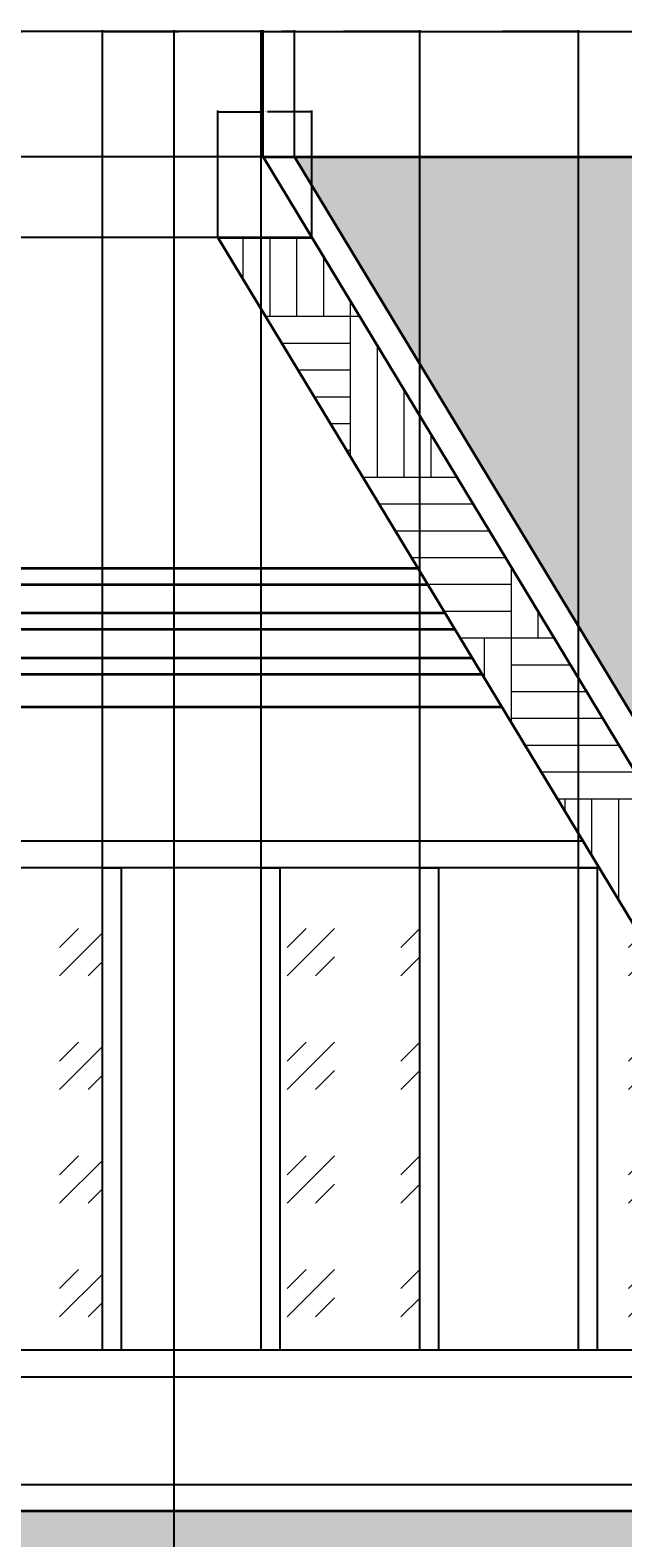
# Model space of a CAD drawing. Units: inches. Extents: x -9 to 389, y -55 to 344.
# Tile 4 of 5: x 133 to 221, y 119 to 344. Entities that reach past the tile are written whole.
import ezdxf

# ---------------------------------------------------------------- set-up
doc = ezdxf.new("R2010")
doc.units = ezdxf.units.IN
doc.header["$MEASUREMENT"] = 0
for name, color, linetype, lineweight in [('A-ANNO-DIMS', 2, 'Continuous', 18), ('A-ELEV', 7, 'Continuous', 35), ('A-ELEV-PATT', 8, 'Continuous', 13), ('A-GLAZ', 4, 'Continuous', 25), ('A-GLAZ-PATT', 252, 'Continuous', 13), ('A-ROOF', 1, 'Continuous', 35), ('A-ROOF-PATT', 8, 'Continuous', 13)]:
    doc.layers.add(name, color=color, linetype=linetype, lineweight=lineweight)
doc.styles.get("Standard").update_dxf_attribs({"font": 'arial.ttf'})
doc.dimstyles.get("Standard").update_dxf_attribs({"dimtxt": 0.18, "dimasz": 0.18, "dimexe": 0.18, "dimexo": 0.0625, "dimgap": 0.09, "dimtad": 0, "dimtih": 1, "dimtoh": 1, "dimdec": 4, "dimzin": 0, "dimdsep": 46, "dimtxsty": 'Standard', "dimcen": 0.09, "dimadec": 0, "dimazin": 0, "dimtfac": 1, "dimtdec": 4, "dimtofl": 0, "dimtmove": 0, "dimatfit": 3, "dimfxl": 1, "dimtolj": 1, "dimtzin": 0, "dimarcsym": 0})

# ---------------------------------------------------------------- blocks, each defined once
blk = doc.blocks.new('*D4')
at = {"layer": 'A-ANNO-DIMS', "color": 0, "lineweight": -2, "transparency": 16777216}
for p, q in [((71.45, 157.47), (71.45, 343.8)), ((71.63, 343.62), (119.03, 343.62)), ((167.08, 343.62), (119.68, 343.62)), ((167.26, 324.93), (167.26, 343.8))]:
    blk.add_line(p, q, dxfattribs=at)
at = {"layer": 'A-ANNO-DIMS', "color": 0, "transparency": 16777216}
for points in [[(71.63, 343.65), (71.63, 343.59), (71.45, 343.62)], [(167.08, 343.65), (167.08, 343.59), (167.26, 343.62)]]:
    blk.add_solid(points, dxfattribs=at)
at = {"layer": 'Defpoints', "color": 0, "transparency": 16777216}
for p in [(167.26, 343.62), (167.26, 324.87), (71.45, 157.4)]:
    blk.add_point(p, dxfattribs=at)
at = {"layer": 'A-ANNO-DIMS', "color": 0, "transparency": 16777216, "insert": (119.35, 343.62), "char_height": 0.18, "attachment_point": 5}
blk.add_mtext('\\A1;95.8', dxfattribs=at)
blk = doc.blocks.new('*D5')
at = {"layer": 'A-ANNO-DIMS', "color": 0, "lineweight": -2, "transparency": 16777216}
for p, q in [((167.26, 324.93), (167.26, 343.8)), ((167.44, 343.62), (169.2, 343.62)), ((171.75, 343.62), (169.99, 343.62)), ((171.93, 324.93), (171.93, 343.8))]:
    blk.add_line(p, q, dxfattribs=at)
at = {"layer": 'A-ANNO-DIMS', "color": 0, "transparency": 16777216}
for points in [[(167.44, 343.65), (167.44, 343.59), (167.26, 343.62)], [(171.75, 343.65), (171.75, 343.59), (171.93, 343.62)]]:
    blk.add_solid(points, dxfattribs=at)
at = {"layer": 'Defpoints', "color": 0, "transparency": 16777216}
for p in [(171.93, 343.62), (167.26, 324.87), (171.93, 324.87)]:
    blk.add_point(p, dxfattribs=at)
at = {"layer": 'A-ANNO-DIMS', "color": 0, "transparency": 16777216, "insert": (169.59, 343.62), "char_height": 0.18, "attachment_point": 5}
blk.add_mtext('\\A1;4.674', dxfattribs=at)
blk = doc.blocks.new('*D6')
at = {"layer": 'A-ANNO-DIMS', "color": 0, "lineweight": -2, "transparency": 16777216}
for p, q in [((171.93, 324.93), (171.93, 343.8)), ((172.11, 343.62), (270.34, 343.62)), ((369.47, 343.62), (271.25, 343.62)), ((369.65, 324.93), (369.65, 343.8))]:
    blk.add_line(p, q, dxfattribs=at)
at = {"layer": 'A-ANNO-DIMS', "color": 0, "transparency": 16777216}
for points in [[(172.11, 343.65), (172.11, 343.59), (171.93, 343.62)], [(369.47, 343.65), (369.47, 343.59), (369.65, 343.62)]]:
    blk.add_solid(points, dxfattribs=at)
at = {"layer": 'Defpoints', "color": 0, "transparency": 16777216}
for p in [(369.65, 343.62), (171.93, 324.87), (369.65, 324.87)]:
    blk.add_point(p, dxfattribs=at)
at = {"layer": 'A-ANNO-DIMS', "color": 0, "transparency": 16777216, "insert": (270.79, 343.62), "char_height": 0.18, "attachment_point": 5}
blk.add_mtext('\\A1;197.72', dxfattribs=at)
blk = doc.blocks.new('*D19')
at = {"layer": 'A-ANNO-DIMS', "color": 0, "lineweight": -2, "transparency": 16777216}
for p, q in [((66.21, 14.83), (66.21, 343.8)), ((66.39, 343.62), (109.71, 343.62)), ((153.81, 343.62), (110.5, 343.62)), ((153.99, 14.83), (153.99, 343.8))]:
    blk.add_line(p, q, dxfattribs=at)
at = {"layer": 'A-ANNO-DIMS', "color": 0, "transparency": 16777216}
for points in [[(66.39, 343.65), (66.39, 343.59), (66.21, 343.62)], [(153.81, 343.65), (153.81, 343.59), (153.99, 343.62)]]:
    blk.add_solid(points, dxfattribs=at)
at = {"layer": 'Defpoints', "color": 0, "transparency": 16777216}
for p in [(153.99, 343.62), (66.21, 14.77), (153.99, 14.77)]:
    blk.add_point(p, dxfattribs=at)
at = {"layer": 'A-ANNO-DIMS', "color": 0, "transparency": 16777216, "insert": (110.1, 343.62), "char_height": 0.18, "attachment_point": 5}
blk.add_mtext('\\A1;87.77', dxfattribs=at)
blk = doc.blocks.new('*D20')
at = {"layer": 'A-ANNO-DIMS', "color": 0, "lineweight": -2, "transparency": 16777216}
for p, q in [((369.72, 324.87), (388.58, 324.87)), ((388.4, 324.69), (388.4, 144.62)), ((388.4, -35.81), (388.4, 144.26)), ((146.92, -35.99), (388.58, -35.99))]:
    blk.add_line(p, q, dxfattribs=at)
at = {"layer": 'A-ANNO-DIMS', "color": 0, "transparency": 16777216}
for points in [[(388.37, 324.69), (388.43, 324.69), (388.4, 324.87)], [(388.37, -35.81), (388.43, -35.81), (388.4, -35.99)]]:
    blk.add_solid(points, dxfattribs=at)
at = {"layer": 'Defpoints', "color": 0, "transparency": 16777216}
for p in [(369.65, 324.87), (388.4, 324.87), (146.86, -35.99)]:
    blk.add_point(p, dxfattribs=at)
at = {"layer": 'A-ANNO-DIMS', "color": 0, "transparency": 16777216, "insert": (388.4, 144.44), "char_height": 0.18, "attachment_point": 5}
blk.add_mtext('\\A1;360.86', dxfattribs=at)
blk = doc.blocks.new('*D28')
at = {"layer": 'A-ANNO-DIMS', "color": 0, "lineweight": -2, "transparency": 16777216}
for p, q in [((160.42, 312.87), (-9.28, 312.87)), ((-9.1, 312.69), (-9.1, 297.72)), ((-9.1, 282.38), (-9.1, 297.35)), ((9.59, 282.2), (-9.28, 282.2))]:
    blk.add_line(p, q, dxfattribs=at)
at = {"layer": 'A-ANNO-DIMS', "color": 0, "transparency": 16777216}
for points in [[(-9.13, 312.69), (-9.07, 312.69), (-9.1, 312.87)], [(-9.13, 282.38), (-9.07, 282.38), (-9.1, 282.2)]]:
    blk.add_solid(points, dxfattribs=at)
at = {"layer": 'Defpoints', "color": 0, "transparency": 16777216}
for p in [(-9.1, 312.87), (160.49, 312.87), (9.65, 282.2)]:
    blk.add_point(p, dxfattribs=at)
at = {"layer": 'A-ANNO-DIMS', "color": 0, "transparency": 16777216, "insert": (-9.1, 297.54), "char_height": 0.18, "attachment_point": 5}
blk.add_mtext('\\A1;30.67', dxfattribs=at)
blk = doc.blocks.new('*D29')
at = {"layer": 'A-ANNO-DIMS', "color": 0, "lineweight": -2, "transparency": 16777216}
for p, q in [((369.59, 324.87), (-9.28, 324.87)), ((-9.1, 324.69), (-9.1, 319.05)), ((-9.1, 313.05), (-9.1, 318.69)), ((160.42, 312.87), (-9.28, 312.87))]:
    blk.add_line(p, q, dxfattribs=at)
at = {"layer": 'A-ANNO-DIMS', "color": 0, "transparency": 16777216}
for points in [[(-9.13, 324.69), (-9.07, 324.69), (-9.1, 324.87)], [(-9.13, 313.05), (-9.07, 313.05), (-9.1, 312.87)]]:
    blk.add_solid(points, dxfattribs=at)
at = {"layer": 'Defpoints', "color": 0, "transparency": 16777216}
for p in [(-9.1, 324.87), (369.65, 324.87), (160.49, 312.87)]:
    blk.add_point(p, dxfattribs=at)
at = {"layer": 'A-ANNO-DIMS', "color": 0, "transparency": 16777216, "insert": (-9.1, 318.87), "char_height": 0.18, "attachment_point": 5}
blk.add_mtext('\\A1;12', dxfattribs=at)
blk = doc.blocks.new('*D38')
at = {"layer": 'A-ANNO-DIMS', "color": 0, "lineweight": -2, "transparency": 16777216}
for p, q in [((160.49, 312.93), (160.49, 331.8)), ((160.67, 331.62), (167.11, 331.62)), ((174.33, 331.62), (167.88, 331.62)), ((174.51, 312.93), (174.51, 331.8))]:
    blk.add_line(p, q, dxfattribs=at)
at = {"layer": 'A-ANNO-DIMS', "color": 0, "transparency": 16777216}
for points in [[(160.67, 331.65), (160.67, 331.59), (160.49, 331.62)], [(174.33, 331.65), (174.33, 331.59), (174.51, 331.62)]]:
    blk.add_solid(points, dxfattribs=at)
at = {"layer": 'Defpoints', "color": 0, "transparency": 16777216}
for p in [(174.51, 331.62), (160.49, 312.87), (174.51, 312.87)]:
    blk.add_point(p, dxfattribs=at)
at = {"layer": 'A-ANNO-DIMS', "color": 0, "transparency": 16777216, "insert": (167.5, 331.62), "char_height": 0.18, "attachment_point": 5}
blk.add_mtext('\\A1;14.02', dxfattribs=at)
blk = doc.blocks.new('*D58')
at = {"layer": 'A-ANNO-DIMS', "color": 0, "lineweight": -2, "transparency": 16777216}
for p, q in [((120.3, 146.83), (120.3, 343.8)), ((120.48, 343.62), (131.33, 343.62)), ((143.12, 343.62), (132.26, 343.62)), ((143.3, 146.83), (143.3, 343.8))]:
    blk.add_line(p, q, dxfattribs=at)
at = {"layer": 'A-ANNO-DIMS', "color": 0, "transparency": 16777216}
for points in [[(120.48, 343.65), (120.48, 343.59), (120.3, 343.62)], [(143.12, 343.65), (143.12, 343.59), (143.3, 343.62)]]:
    blk.add_solid(points, dxfattribs=at)
at = {"layer": 'Defpoints', "color": 0, "transparency": 16777216}
for p in [(143.3, 343.62), (120.3, 146.77), (143.3, 146.77)]:
    blk.add_point(p, dxfattribs=at)
at = {"layer": 'A-ANNO-DIMS', "color": 0, "transparency": 16777216, "insert": (131.8, 343.62), "char_height": 0.18, "attachment_point": 5}
blk.add_mtext('\\A1;22.994', dxfattribs=at)
blk = doc.blocks.new('*D59')
at = {"layer": 'A-ANNO-DIMS', "color": 0, "lineweight": -2, "transparency": 16777216}
for p, q in [((143.3, 146.83), (143.3, 343.8)), ((143.48, 343.62), (154.66, 343.62)), ((166.78, 343.62), (155.59, 343.62)), ((166.96, 146.83), (166.96, 343.8))]:
    blk.add_line(p, q, dxfattribs=at)
at = {"layer": 'A-ANNO-DIMS', "color": 0, "transparency": 16777216}
for points in [[(143.48, 343.65), (143.48, 343.59), (143.3, 343.62)], [(166.78, 343.65), (166.78, 343.59), (166.96, 343.62)]]:
    blk.add_solid(points, dxfattribs=at)
at = {"layer": 'Defpoints', "color": 0, "transparency": 16777216}
for p in [(166.96, 343.62), (143.3, 146.77), (166.96, 146.77)]:
    blk.add_point(p, dxfattribs=at)
at = {"layer": 'A-ANNO-DIMS', "color": 0, "transparency": 16777216, "insert": (155.13, 343.62), "char_height": 0.18, "attachment_point": 5}
blk.add_mtext('\\A1;23.666', dxfattribs=at)
blk = doc.blocks.new('*D60')
at = {"layer": 'A-ANNO-DIMS', "color": 0, "lineweight": -2, "transparency": 16777216}
for p, q in [((166.96, 146.83), (166.96, 343.8)), ((167.14, 343.62), (178.33, 343.62)), ((190.45, 343.62), (179.26, 343.62)), ((190.63, 146.83), (190.63, 343.8))]:
    blk.add_line(p, q, dxfattribs=at)
at = {"layer": 'A-ANNO-DIMS', "color": 0, "transparency": 16777216}
for points in [[(167.14, 343.65), (167.14, 343.59), (166.96, 343.62)], [(190.45, 343.65), (190.45, 343.59), (190.63, 343.62)]]:
    blk.add_solid(points, dxfattribs=at)
at = {"layer": 'Defpoints', "color": 0, "transparency": 16777216}
for p in [(190.63, 343.62), (166.96, 146.77), (190.63, 146.77)]:
    blk.add_point(p, dxfattribs=at)
at = {"layer": 'A-ANNO-DIMS', "color": 0, "transparency": 16777216, "insert": (178.79, 343.62), "char_height": 0.18, "attachment_point": 5}
blk.add_mtext('\\A1;23.666', dxfattribs=at)
blk = doc.blocks.new('*D61')
at = {"layer": 'A-ANNO-DIMS', "color": 0, "lineweight": -2, "transparency": 16777216}
for p, q in [((190.63, 146.83), (190.63, 343.8)), ((190.81, 343.62), (201.99, 343.62)), ((214.11, 343.62), (202.92, 343.62)), ((214.29, 146.83), (214.29, 343.8))]:
    blk.add_line(p, q, dxfattribs=at)
at = {"layer": 'A-ANNO-DIMS', "color": 0, "transparency": 16777216}
for points in [[(190.81, 343.65), (190.81, 343.59), (190.63, 343.62)], [(214.11, 343.65), (214.11, 343.59), (214.29, 343.62)]]:
    blk.add_solid(points, dxfattribs=at)
at = {"layer": 'Defpoints', "color": 0, "transparency": 16777216}
for p in [(214.29, 343.62), (190.63, 146.77), (214.29, 146.77)]:
    blk.add_point(p, dxfattribs=at)
at = {"layer": 'A-ANNO-DIMS', "color": 0, "transparency": 16777216, "insert": (202.46, 343.62), "char_height": 0.18, "attachment_point": 5}
blk.add_mtext('\\A1;23.666', dxfattribs=at)
blk = doc.blocks.new('*D62')
at = {"layer": 'A-ANNO-DIMS', "color": 0, "lineweight": -2, "transparency": 16777216}
for p, q in [((214.29, 146.83), (214.29, 343.8)), ((214.47, 343.62), (225.66, 343.62)), ((237.78, 343.62), (226.59, 343.62)), ((237.96, 146.83), (237.96, 343.8))]:
    blk.add_line(p, q, dxfattribs=at)
at = {"layer": 'A-ANNO-DIMS', "color": 0, "transparency": 16777216}
for points in [[(214.47, 343.65), (214.47, 343.59), (214.29, 343.62)], [(237.78, 343.65), (237.78, 343.59), (237.96, 343.62)]]:
    blk.add_solid(points, dxfattribs=at)
at = {"layer": 'Defpoints', "color": 0, "transparency": 16777216}
for p in [(237.96, 343.62), (214.29, 146.77), (237.96, 146.77)]:
    blk.add_point(p, dxfattribs=at)
at = {"layer": 'A-ANNO-DIMS', "color": 0, "transparency": 16777216, "insert": (226.12, 343.62), "char_height": 0.18, "attachment_point": 5}
blk.add_mtext('\\A1;23.666', dxfattribs=at)
blk = doc.blocks.new('*D64')
at = {"layer": 'A-ANNO-DIMS', "color": 0, "lineweight": -2, "transparency": 16777216}
for p, q in [((130.27, 126.74), (388.58, 126.74)), ((388.4, 126.56), (388.4, 124.94)), ((388.4, 122.95), (388.4, 124.57)), ((118.84, 122.77), (388.58, 122.77))]:
    blk.add_line(p, q, dxfattribs=at)
at = {"layer": 'A-ANNO-DIMS', "color": 0, "transparency": 16777216}
for points in [[(388.37, 126.56), (388.43, 126.56), (388.4, 126.74)], [(388.37, 122.95), (388.43, 122.95), (388.4, 122.77)]]:
    blk.add_solid(points, dxfattribs=at)
at = {"layer": 'Defpoints', "color": 0, "transparency": 16777216}
for p in [(130.2, 126.74), (388.4, 126.74), (118.78, 122.77)]:
    blk.add_point(p, dxfattribs=at)
at = {"layer": 'A-ANNO-DIMS', "color": 0, "transparency": 16777216, "insert": (388.4, 124.76), "char_height": 0.18, "attachment_point": 5}
blk.add_mtext('\\A1;3.976', dxfattribs=at)
blk = doc.blocks.new('*D68')
at = {"layer": 'A-ANNO-DIMS', "color": 0, "lineweight": -2, "transparency": 16777216}
for p, q in [((114.32, 122.71), (114.32, -54.92)), ((289.4, 122.71), (289.4, -54.92)), ((114.5, -54.74), (201.4, -54.74)), ((289.22, -54.74), (202.31, -54.74))]:
    blk.add_line(p, q, dxfattribs=at)
at = {"layer": 'A-ANNO-DIMS', "color": 0, "transparency": 16777216}
for points in [[(114.5, -54.71), (114.5, -54.77), (114.32, -54.74)], [(289.22, -54.71), (289.22, -54.77), (289.4, -54.74)]]:
    blk.add_solid(points, dxfattribs=at)
at = {"layer": 'Defpoints', "color": 0, "transparency": 16777216}
for p in [(114.32, 122.77), (289.4, 122.77), (289.4, -54.74)]:
    blk.add_point(p, dxfattribs=at)
at = {"layer": 'A-ANNO-DIMS', "color": 0, "transparency": 16777216, "insert": (201.86, -54.74), "char_height": 0.18, "attachment_point": 5}
blk.add_mtext('\\A1;175.08', dxfattribs=at)

msp = doc.modelspace()

# ---------------------------------------------------------------- hatches: boundary and pattern name
at = {"layer": 'A-ELEV-PATT'}
h = msp.add_hatch(color=256, dxfattribs=at)
h.dxf.hatch_style = 1
h.paths.add_polyline_path([(369.6533, 324.8713), (171.9292, 324.8713), (224.4434, 237.9774), (369.6533, 237.9774)])
h.paths.add_polyline_path([(369.6533, 224.3149), (232.7004, 224.3149), (294.07, 122.7681), (369.6533, 122.7681)])
h = msp.add_hatch(color=256, dxfattribs=at)
h.dxf.hatch_style = 1
h.paths.add_polyline_path([(369.6533, 122.7681), (289.3963, 122.7681), (9.6533, 122.7681), (9.6533, 2.7681), (369.6533, 2.7681)])
h.paths.add_polyline_path([(177.6533, 110.7681), (177.6533, 14.7681), (21.6533, 14.7681), (21.6533, 110.7681)], flags=16)
h.paths.add_polyline_path([(201.6533, 110.7681), (357.6533, 110.7681), (357.6533, 14.7681), (201.6533, 14.7681)], flags=16)
h.paths.add_polyline_path([(156.7573, 110.7681), (156.7573, 14.7681), (153.9877, 14.7681), (153.9877, 110.7681)], flags=0)
h.paths.add_polyline_path([(222.5492, 110.7681), (225.3188, 110.7681), (225.3188, 14.7681), (222.5492, 14.7681)], flags=0)
h.paths.add_polyline_path([(246.2148, 110.7681), (248.9844, 110.7681), (248.9844, 14.7681), (246.2148, 14.7681)], flags=0)
h.paths.add_polyline_path([(269.8803, 110.7681), (272.65, 110.7681), (272.65, 14.7681), (269.8803, 14.7681)], flags=0)
h.paths.add_polyline_path([(68.9844, 110.7681), (68.9844, 14.7681), (66.2148, 14.7681), (66.2148, 110.7681)], flags=0)
h.paths.add_polyline_path([(45.3188, 110.7681), (45.3188, 14.7681), (42.5492, 14.7681), (42.5492, 110.7681)], flags=0)
at = {"layer": 'A-GLAZ-PATT', "transparency": 33554536}
h = msp.add_hatch(dxfattribs=at)
h.set_pattern_fill('GOST_GLASS', color=256, scale=2)
h.set_pattern_definition([(45, (-83.729, -34.93), (16.97056, 0), [10, -14]), (45, (-79.486, -34.93), (16.97056, 0), [4, -20]), (45, (-83.729, -30.687), (16.97056, 0), [4, -20])])
h.paths.add_polyline_path([(153.9877, 110.7681), (68.9844, 110.7681), (68.9844, 14.7681), (153.9877, 14.7681)])
h.paths.add_polyline_path([(357.6533, 110.7681), (272.65, 110.7681), (272.65, 14.7681), (357.6533, 14.7681)])
h.paths.add_polyline_path([(190.6266, 218.7681), (169.7307, 218.7681), (169.7307, 146.7681), (190.6266, 146.7681)])
h.paths.add_polyline_path([(143.2954, 218.7681), (122.3995, 218.7681), (122.3995, 146.7681), (143.2954, 146.7681)])
h.paths.add_polyline_path([(237.9578, 184.6816), (217.3576, 218.7681), (217.0618, 218.7681), (217.0618, 146.7681), (237.9578, 146.7681)])
h.paths.add_polyline_path([(42.5492, 110.7681), (21.6533, 110.7681), (21.6533, 14.7681), (42.5492, 14.7681)])
h.paths.add_polyline_path([(246.2148, 110.7681), (225.3188, 110.7681), (225.3188, 14.7681), (246.2148, 14.7681)])
at = {"layer": 'A-ROOF-PATT'}
h = msp.add_hatch(dxfattribs=at)
h.set_pattern_fill('AR-PARQ1', color=256, scale=2)
h.set_pattern_definition([(90, (-83.73, -34.93), (-24, 24), [24, -24]), (90, (-79.73, -34.93), (-24, 24), [24, -24]), (90, (-75.73, -34.93), (-24, 24), [24, -24]), (90, (-71.73, -34.93), (-24, 24), [24, -24]), (90, (-67.73, -34.93), (-24, 24), [24, -24]), (90, (-63.73, -34.93), (-24, 24), [24, -24]), (90, (-59.73, -34.93), (-24, 24), [24, -24]), (0, (-83.73, -10.93), (24, -24), [24, -24]), (0, (-83.73, -6.93), (24, -24), [24, -24]), (0, (-83.73, -2.93), (24, -24), [24, -24]), (0, (-83.73, 1.07), (24, -24), [24, -24]), (0, (-83.73, 5.07), (24, -24), [24, -24]), (0, (-83.73, 9.07), (24, -24), [24, -24]), (0, (-83.73, 13.07), (24, -24), [24, -24])])
h.paths.add_polyline_path([(59.2615, 270.2003), (45.8744, 270.2003), (116.6802, 127.0192), (130.2035, 126.7437)])
h.paths.add_polyline_path([(174.5076, 312.8713), (160.4864, 312.8713), (271.5791, 129.0492), (285.7644, 128.7778)])

# ---------------------------------------------------------------- linework, layer by layer
at = {"layer": 'A-ELEV'}
for p, q in [((202.8532, 242.7681), (72.8272, 242.7681)), ((369.6533, 122.7681), (9.6533, 122.7681))]:
    msp.add_line(p, q, dxfattribs=at)
for points in [[(62.5664, 263.5172), (190.3135, 263.5172)], [(191.8259, 261.0148), (191.8259, 261.0148), (63.8039, 261.0148)], [(65.8726, 256.8316), (194.354, 256.8316)], [(195.8663, 254.3292), (195.8663, 254.3292), (67.1101, 254.3292)], [(69.1949, 250.1134), (198.4141, 250.1134)], [(199.9265, 247.611), (199.9265, 247.611), (70.4324, 247.611)]]:
    msp.add_lwpolyline(points, dxfattribs=at)
at = {"layer": 'A-GLAZ'}
for p, q in [((214.9402, 222.7681), (82.7176, 222.7681)), ((217.3576, 218.7681), (84.6957, 218.7681)), ((260.8707, 146.7681), (120.3011, 146.7681)), ((263.2881, 142.7681), (122.2791, 142.7681))]:
    msp.add_line(p, q, dxfattribs=at)
for points in [[(143.2954, 146.7681), (143.2954, 218.7681), (146.0651, 218.7681), (146.0651, 146.7681)], [(166.961, 146.7681), (166.961, 218.7681), (169.7307, 218.7681), (169.7307, 146.7681)], [(190.6266, 146.7681), (190.6266, 218.7681), (193.3963, 218.7681), (193.3963, 146.7681)], [(214.2922, 146.7681), (214.2922, 218.7681), (217.0618, 218.7681), (217.0618, 146.7681)], [(146.0651, 122.7681), (143.2954, 122.7681)], [(169.7307, 122.7681), (166.961, 122.7681)], [(193.3963, 122.7681), (190.6266, 122.7681)], [(217.0618, 122.7681), (214.2922, 122.7681)]]:
    msp.add_lwpolyline(points, dxfattribs=at)
at = {"layer": 'A-ROOF'}
for p, q in [((289.3963, 122.7681), (167.2555, 324.8713)), ((167.2555, 324.8713), (369.6533, 324.8713)), ((294.07, 122.7681), (171.9292, 324.8713)), ((271.5791, 129.0492), (160.4864, 312.8713)), ((160.4864, 312.8713), (174.5076, 312.8713))]:
    msp.add_line(p, q, dxfattribs=at)

# ---------------------------------------------------------------- dimensions: what is measured, and where the dimension line sits
at = {"layer": 'A-ANNO-DIMS'}
for base, p1, p2, override, picture, middle in [((153.9877, 343.6213), (66.2148, 14.7681), (153.9877, 14.7681), {"dimdec": 2, "dimlfac": 1, "dimrnd": 0, "dimzin": 0, "dimdsep": 46, "dimlunit": 2}, '*D19', (110.1012, 343.6213)), ((167.2555, 343.6213), (71.4494, 157.4044), (167.2555, 324.8713), {"dimdec": 1, "dimlfac": 1, "dimrnd": 0, "dimzin": 0, "dimdsep": 46, "dimlunit": 2}, '*D4', (119.3525, 343.6213)), ((143.2954, 343.6213), (120.3011, 146.7681), (143.2954, 146.7681), {"dimdec": 3, "dimlfac": 1, "dimrnd": 0, "dimzin": 0, "dimdsep": 46, "dimlunit": 2}, '*D58', (131.7983, 343.6213)), ((166.961, 343.6213), (143.2954, 146.7681), (166.961, 146.7681), {"dimdec": 3, "dimlfac": 1, "dimrnd": 0, "dimzin": 0, "dimdsep": 46, "dimlunit": 2}, '*D59', (155.1282, 343.6213)), ((190.6266, 343.6213), (166.961, 146.7681), (190.6266, 146.7681), {"dimdec": 3, "dimlfac": 1, "dimrnd": 0, "dimzin": 0, "dimdsep": 46, "dimlunit": 2}, '*D60', (178.7938, 343.6213)), ((171.9292, 343.6213), (167.2555, 324.8713), (171.9292, 324.8713), {"dimdec": 3, "dimlfac": 1, "dimrnd": 0, "dimzin": 0, "dimdsep": 46, "dimlunit": 2}, '*D5', (169.5923, 343.6213)), ((369.6533, 343.6213), (171.9292, 324.8713), (369.6533, 324.8713), {"dimdec": 2, "dimlfac": 1, "dimrnd": 0, "dimzin": 0, "dimdsep": 46, "dimlunit": 2}, '*D6', (270.7912, 343.6213)), ((214.2922, 343.6213), (190.6266, 146.7681), (214.2922, 146.7681), {"dimdec": 3, "dimlfac": 1, "dimrnd": 0, "dimzin": 0, "dimdsep": 46, "dimlunit": 2}, '*D61', (202.4594, 343.6213)), ((237.9578, 343.6213), (214.2922, 146.7681), (237.9578, 146.7681), {"dimdec": 3, "dimlfac": 1, "dimrnd": 0, "dimzin": 0, "dimdsep": 46, "dimlunit": 2}, '*D62', (226.125, 343.6213)), ((174.5076, 331.6213), (160.4864, 312.8713), (174.5076, 312.8713), {"dimdec": 2, "dimlfac": 1, "dimrnd": 0, "dimzin": 0, "dimdsep": 46, "dimlunit": 2}, '*D38', (167.497, 331.6213)), ((289.3963, -54.7386), (114.32, 122.7681), (289.3963, 122.7681), {"dimdec": 2, "dimlfac": 1, "dimrnd": 0, "dimzin": 0, "dimdsep": 46, "dimlunit": 2}, '*D68', (201.8582, -54.7386))]:
    dim = msp.add_linear_dim(base=base, p1=p1, p2=p2, dimstyle='Standard', override=override, dxfattribs=at)
    dim.commit()
    dim.dimension.update_dxf_attribs({"geometry": picture, "text_midpoint": middle})
for base, p1, p2, override, picture, middle in [((-9.0967, 324.8713), (160.4864, 312.8713), (369.6533, 324.8713), {"dimdec": 0, "dimlfac": 1, "dimrnd": 0, "dimzin": 0, "dimdsep": 46, "dimlunit": 2}, '*D29', (-9.0967, 318.8713)), ((388.4033, 324.8713), (146.8603, -35.9886), (369.6533, 324.8713), {"dimdec": 2, "dimlfac": 1, "dimrnd": 0, "dimzin": 0, "dimdsep": 46, "dimlunit": 2}, '*D20', (388.4033, 144.4414)), ((-9.0967, 312.8713), (9.6533, 282.2003), (160.4864, 312.8713), {"dimdec": 2, "dimlfac": 1, "dimrnd": 0, "dimzin": 0, "dimdsep": 46, "dimlunit": 2}, '*D28', (-9.0967, 297.5358)), ((388.4033, 126.7437), (118.7824, 122.7681), (130.2035, 126.7437), {"dimdec": 3, "dimlfac": 1, "dimrnd": 0, "dimzin": 0, "dimdsep": 46, "dimlunit": 2}, '*D64', (388.4033, 124.7559))]:
    dim = msp.add_linear_dim(base=base, p1=p1, p2=p2, angle=90, dimstyle='Standard', override=override, dxfattribs=at)
    dim.commit()
    dim.dimension.update_dxf_attribs({"geometry": picture, "text_midpoint": middle})

doc.saveas('drawing.dxf')
